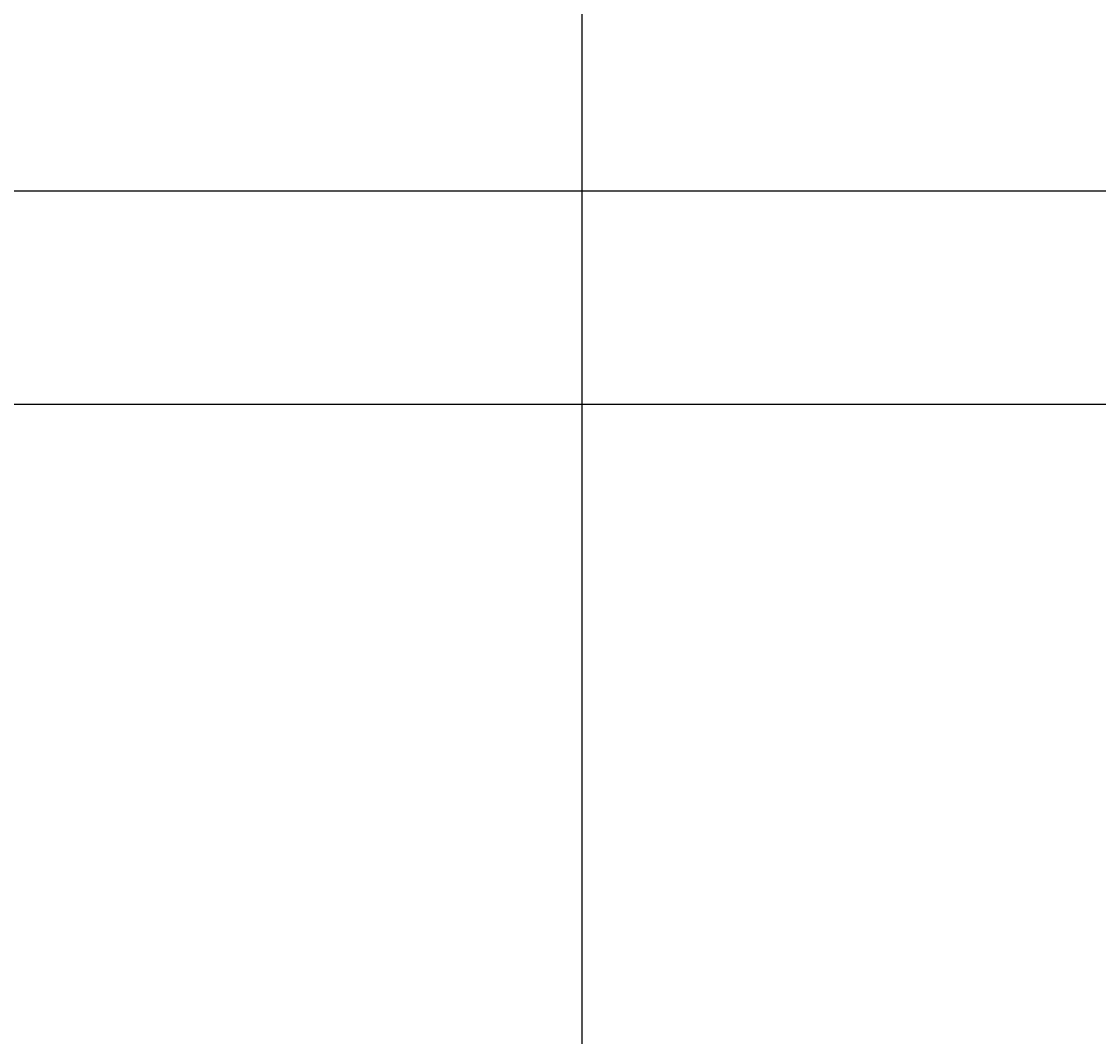
# Model space of a CAD drawing. Units: inches. Extents: x 35362 to 73946, y 43607 to 67532.
# Tile 75 of 134: x 49711 to 50119, y 47304 to 47689. Entities that reach past the tile are written whole.
import ezdxf

# ---------------------------------------------------------------- set-up
doc = ezdxf.new("R2010")
doc.units = ezdxf.units.IN
doc.header["$MEASUREMENT"] = 0
doc.layers.add('A-ANNO-DIMS', color=2, linetype='Continuous', lineweight=18)
doc.styles.get("Standard").update_dxf_attribs({"font": 'arial.ttf'})
doc.dimstyles.get("Standard").update_dxf_attribs({"dimtxt": 0.18, "dimasz": 0.18, "dimexe": 0.18, "dimexo": 0.0625, "dimgap": 0.09, "dimtad": 0, "dimtih": 1, "dimtoh": 1, "dimdec": 4, "dimzin": 0, "dimdsep": 46, "dimtxsty": 'Standard', "dimcen": 0.09, "dimadec": 0, "dimazin": 0, "dimtfac": 1, "dimtdec": 4, "dimtofl": 0, "dimtmove": 0, "dimatfit": 3, "dimfxl": 1, "dimtolj": 1, "dimtzin": 0, "dimarcsym": 0})

# ---------------------------------------------------------------- blocks, each defined once
blk = doc.blocks.new('*D11')
at = {"layer": 'A-ANNO-DIMS', "color": 0, "lineweight": -2, "transparency": 16777216}
for p, q in [((47978.66, 56028.77), (47978.66, 43606.68)), ((53109.76, 56028.77), (53109.76, 43606.68)), ((47978.84, 43606.86), (50543.87, 43606.86)), ((53109.58, 43606.86), (50544.55, 43606.86))]:
    blk.add_line(p, q, dxfattribs=at)
at = {"layer": 'A-ANNO-DIMS', "color": 0, "transparency": 16777216}
for points in [[(47978.84, 43606.89), (47978.84, 43606.83), (47978.66, 43606.86)], [(53109.58, 43606.89), (53109.58, 43606.83), (53109.76, 43606.86)]]:
    blk.add_solid(points, dxfattribs=at)
at = {"layer": 'Defpoints', "color": 0, "transparency": 16777216}
for p in [(47978.66, 56028.84), (53109.76, 56028.84), (53109.76, 43606.86)]:
    blk.add_point(p, dxfattribs=at)
at = {"layer": 'A-ANNO-DIMS', "color": 0, "transparency": 16777216, "insert": (50544.21, 43606.86), "char_height": 0.18, "attachment_point": 5}
blk.add_mtext('\\A1;5131', dxfattribs=at)
blk = doc.blocks.new('*D13')
at = {"layer": 'A-ANNO-DIMS', "color": 0, "lineweight": -2, "transparency": 16777216}
for p, q in [((48373.49, 51694.02), (48373.49, 43606.68)), ((51029.04, 51694.02), (51029.04, 43606.68)), ((48373.67, 43606.86), (49700.8, 43606.86)), ((51028.86, 43606.86), (49701.73, 43606.86))]:
    blk.add_line(p, q, dxfattribs=at)
at = {"layer": 'A-ANNO-DIMS', "color": 0, "transparency": 16777216}
for points in [[(48373.67, 43606.89), (48373.67, 43606.83), (48373.49, 43606.86)], [(51028.86, 43606.89), (51028.86, 43606.83), (51029.04, 43606.86)]]:
    blk.add_solid(points, dxfattribs=at)
at = {"layer": 'Defpoints', "color": 0, "transparency": 16777216}
for p in [(48373.49, 51694.09), (51029.04, 51694.09), (51029.04, 43606.86)]:
    blk.add_point(p, dxfattribs=at)
at = {"layer": 'A-ANNO-DIMS', "color": 0, "transparency": 16777216, "insert": (49701.27, 43606.86), "char_height": 0.18, "attachment_point": 5}
blk.add_mtext('\\A1;2655.6', dxfattribs=at)
blk = doc.blocks.new('*D17')
at = {"layer": 'A-ANNO-DIMS', "color": 0, "lineweight": -2, "transparency": 16777216}
for p, q in [((49923.31, 61293.22), (49923.31, 43606.68)), ((51913.93, 61293.22), (51913.93, 43606.68)), ((49923.49, 43606.86), (50918.16, 43606.86)), ((51913.75, 43606.86), (50919.07, 43606.86))]:
    blk.add_line(p, q, dxfattribs=at)
at = {"layer": 'A-ANNO-DIMS', "color": 0, "transparency": 16777216}
for points in [[(49923.49, 43606.89), (49923.49, 43606.83), (49923.31, 43606.86)], [(51913.75, 43606.89), (51913.75, 43606.83), (51913.93, 43606.86)]]:
    blk.add_solid(points, dxfattribs=at)
at = {"layer": 'Defpoints', "color": 0, "transparency": 16777216}
for p in [(49923.31, 61293.29), (51913.93, 61293.29), (51913.93, 43606.86)]:
    blk.add_point(p, dxfattribs=at)
at = {"layer": 'A-ANNO-DIMS', "color": 0, "transparency": 16777216, "insert": (50918.62, 43606.86), "char_height": 0.18, "attachment_point": 5}
blk.add_mtext('\\A1;1990.6', dxfattribs=at)
blk = doc.blocks.new('*D43')
at = {"layer": 'A-ANNO-DIMS', "color": 0, "lineweight": -2, "transparency": 16777216}
for p, q in [((62004.67, 47625.18), (35361.77, 47625.18)), ((35361.95, 47625), (35361.95, 47416.9)), ((35361.95, 47208.43), (35361.95, 47416.53)), ((62004.67, 47208.25), (35361.77, 47208.25))]:
    blk.add_line(p, q, dxfattribs=at)
at = {"layer": 'A-ANNO-DIMS', "color": 0, "transparency": 16777216}
for points in [[(35361.92, 47625), (35361.98, 47625), (35361.95, 47625.18)], [(35361.92, 47208.43), (35361.98, 47208.43), (35361.95, 47208.25)]]:
    blk.add_solid(points, dxfattribs=at)
at = {"layer": 'Defpoints', "color": 0, "transparency": 16777216}
for p in [(62004.73, 47625.18), (35361.95, 47208.25), (62004.73, 47208.25)]:
    blk.add_point(p, dxfattribs=at)
at = {"layer": 'A-ANNO-DIMS', "color": 0, "transparency": 16777216, "insert": (35361.95, 47416.72), "char_height": 0.18, "attachment_point": 5}
blk.add_mtext('\\A1;416.9', dxfattribs=at)
blk = doc.blocks.new('*D67')
at = {"layer": 'A-ANNO-DIMS', "color": 0, "lineweight": -2, "transparency": 16777216}
for p, q in [((56873.54, 53351.53), (35361.77, 53351.53)), ((35361.95, 53351.35), (35361.95, 49400.89)), ((35361.95, 45450.07), (35361.95, 49400.53)), ((53793.58, 45449.89), (35361.77, 45449.89))]:
    blk.add_line(p, q, dxfattribs=at)
at = {"layer": 'A-ANNO-DIMS', "color": 0, "transparency": 16777216}
for points in [[(35361.92, 53351.35), (35361.98, 53351.35), (35361.95, 53351.53)], [(35361.92, 45450.07), (35361.98, 45450.07), (35361.95, 45449.89)]]:
    blk.add_solid(points, dxfattribs=at)
at = {"layer": 'Defpoints', "color": 0, "transparency": 16777216}
for p in [(35361.95, 53351.53), (56873.6, 53351.53), (53793.64, 45449.89)]:
    blk.add_point(p, dxfattribs=at)
at = {"layer": 'A-ANNO-DIMS', "color": 0, "transparency": 16777216, "insert": (35361.95, 49400.71), "char_height": 0.18, "attachment_point": 5}
blk.add_mtext('\\A1;7901.6', dxfattribs=at)
blk = doc.blocks.new('*D87')
at = {"layer": 'A-ANNO-DIMS', "color": 0, "lineweight": -2, "transparency": 16777216}
for p, q in [((52362.49, 48318.27), (35361.77, 48318.27)), ((35361.95, 48318.09), (35361.95, 47931.38)), ((35361.95, 47544.31), (35361.95, 47931.02)), ((52362.49, 47544.13), (35361.77, 47544.13))]:
    blk.add_line(p, q, dxfattribs=at)
at = {"layer": 'A-ANNO-DIMS', "color": 0, "transparency": 16777216}
for points in [[(35361.92, 48318.09), (35361.98, 48318.09), (35361.95, 48318.27)], [(35361.92, 47544.31), (35361.98, 47544.31), (35361.95, 47544.13)]]:
    blk.add_solid(points, dxfattribs=at)
at = {"layer": 'Defpoints', "color": 0, "transparency": 16777216}
for p in [(35361.95, 48318.27), (52362.56, 48318.27), (52362.56, 47544.13)]:
    blk.add_point(p, dxfattribs=at)
at = {"layer": 'A-ANNO-DIMS', "color": 0, "transparency": 16777216, "insert": (35361.95, 47931.2), "char_height": 0.18, "attachment_point": 5}
blk.add_mtext('\\A1;774.1', dxfattribs=at)

msp = doc.modelspace()

# ---------------------------------------------------------------- dimensions: what is measured, and where the dimension line sits
at = {"layer": 'A-ANNO-DIMS'}
for base, p1, p2, override, picture, middle in [((51913.931, 43606.859), (49923.307, 61293.286), (51913.931, 61293.286), {"dimdec": 1, "dimlfac": 1, "dimrnd": 0, "dimzin": 0, "dimdsep": 46, "dimlunit": 2}, '*D17', (50918.619, 43606.859)), ((53109.76, 43606.859), (47978.665, 56028.836), (53109.76, 56028.836), {"dimdec": 0, "dimlfac": 1, "dimrnd": 0, "dimzin": 0, "dimdsep": 46, "dimlunit": 2}, '*D11', (50544.212, 43606.859)), ((51029.043, 43606.859), (48373.492, 51694.087), (51029.043, 51694.087), {"dimdec": 1, "dimlfac": 1, "dimrnd": 0, "dimzin": 0, "dimdsep": 46, "dimlunit": 2}, '*D13', (49701.267, 43606.859))]:
    dim = msp.add_linear_dim(base=base, p1=p1, p2=p2, dimstyle='Standard', override=override, dxfattribs=at)
    dim.commit()
    dim.dimension.update_dxf_attribs({"geometry": picture, "text_midpoint": middle})
for base, p1, p2, picture, middle in [((35361.949, 53351.529), (53793.638, 45449.894), (56873.602, 53351.529), '*D67', (35361.949, 49400.712)), ((35361.949, 48318.269), (52362.557, 47544.134), (52362.557, 48318.269), '*D87', (35361.949, 47931.201)), ((35361.949, 47208.25), (62004.728, 47625.181), (62004.728, 47208.25), '*D43', (35361.949, 47416.715))]:
    dim = msp.add_linear_dim(base=base, p1=p1, p2=p2, angle=90, dimstyle='Standard', override={"dimdec": 1, "dimlfac": 1, "dimrnd": 0, "dimzin": 0, "dimdsep": 46, "dimlunit": 2}, dxfattribs=at)
    dim.commit()
    dim.dimension.update_dxf_attribs({"geometry": picture, "text_midpoint": middle})

doc.saveas('drawing.dxf')
